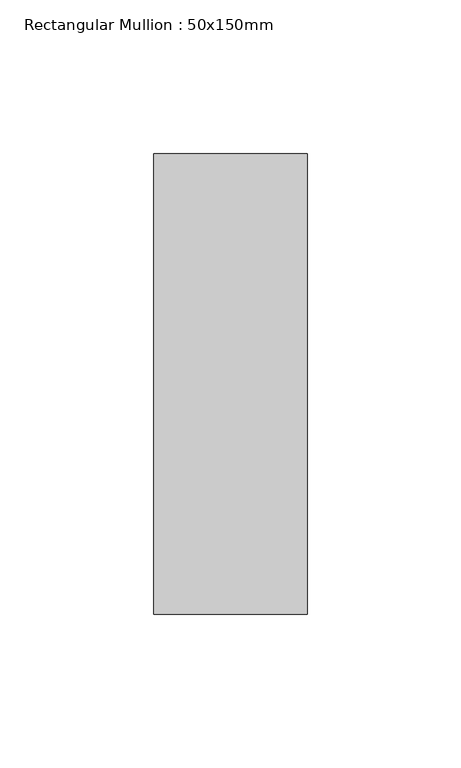
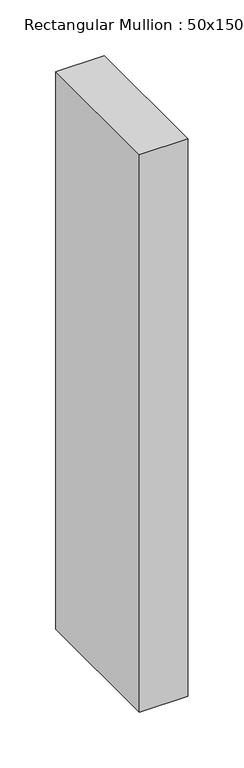
"""IFC4 building model written with IfcOpenShell, lengths in millimetres: member geometry, Rectangular Mullion : 50x150mm."""

from ifc_helpers import new_model, si_unit, frame, origin, place, context, project, spatial, polyline, outline, extrude, source, transform, mapped, element, save


def rectangular_mullion_50x150mm_11f8c00f(model_context):
    return source(origin(), model_context, "Body", "SweptSolid", [
        extrude(outline(polyline([(0.0, 75.0), (0.0, -75.0), (-50.0, -75.0), (-50.0, 75.0), (0.0, 75.0)])), frame((0.0, 0.0, -609.6), z_axis=(0.0, 0.0, 1.0), x_axis=(1.0, 0.0, 0.0)), (0.0, 0.0, 1.0), 609.6),
    ])


if __name__ == "__main__":
    model = new_model("IFC4")
    model_context = context("Model", 3, world=origin())
    ifc_project = project(units=[si_unit("LENGTHUNIT", "METRE", prefix="MILLI")], contexts=[model_context])
    site = spatial("IfcSite", under=ifc_project)
    building = spatial("IfcBuilding", under=site)
    placement = place(None, origin())
    rectangular_mullion_50x150mm_shape = rectangular_mullion_50x150mm_11f8c00f(model_context)
    element("IfcMember", 1, ObjectType="Rectangular Mullion : 50x150mm", at=placement, inside=building, context=model_context, shape_type="MappedRepresentation", body=[
        mapped(rectangular_mullion_50x150mm_shape, transform((0.0, 0.0, 0.0), x_axis=(1.0, 0.0, 0.0), y_axis=(0.0, 1.0, 0.0), z_axis=(0.0, 0.0, 1.0))),
    ])
    save(model, "model.ifc")

# Revit data of these elements
# Type "Rectangular Mullion : 50x150mm"
#   Keynote = "H11"
#   built-in parameter 1007304 = 0.492126 (stored number, unit not read)
#   built-in parameter 1007301 = 0.082021 (stored number, unit not read)
#   built-in parameter 1007300 = 0.082021 (stored number, unit not read)
# Element 1 (IfcMember, "Rectangular Mullion : 50x150mm")
#   Materials on its faces: "Aluminium"
# Materials
#   "Aluminium": class "Metal", colour RGB 247 247 247, transparency 0, Description = "Aluminium 6061", Cost = 0
